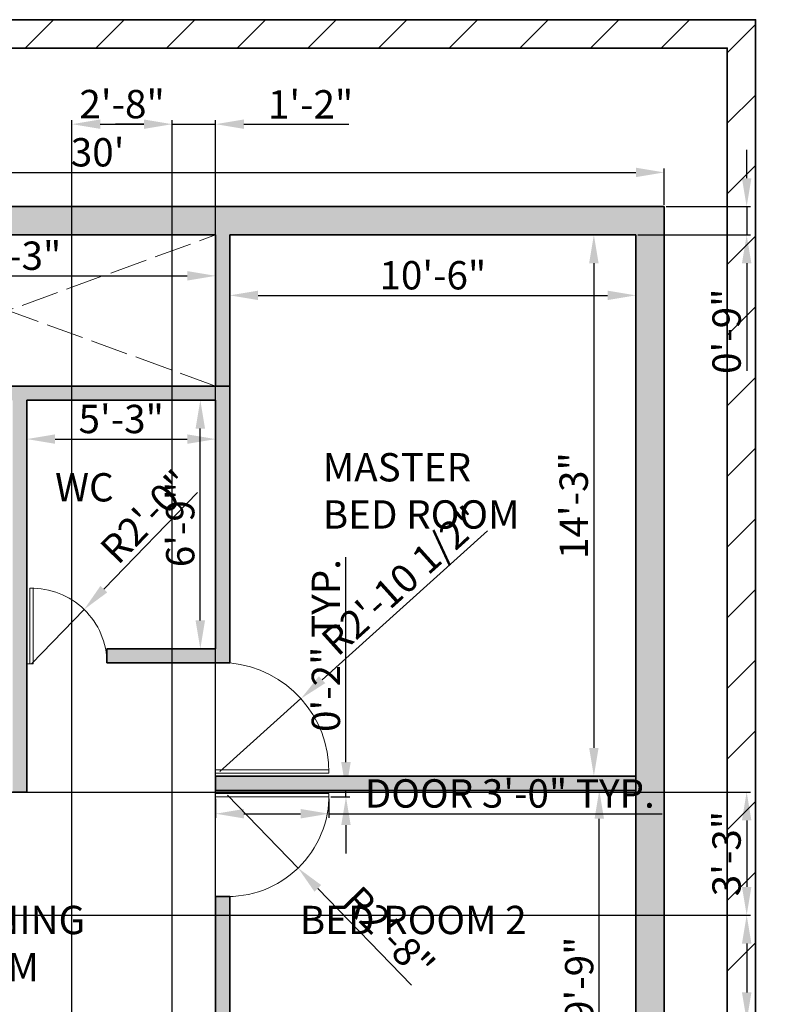
# Model space of a CAD drawing. Units: inches. Extents: x 1130698 to 1131150, y 432269 to 432875.
# Tile 3 of 3: x 1130911 to 1131150, y 432551 to 432864. Entities that reach past the tile are written whole.
import ezdxf

# ---------------------------------------------------------------- set-up
doc = ezdxf.new("R2010")
doc.units = ezdxf.units.IN
doc.linetypes.add('ACAD_ISO02W100', pattern=[15, 12, -3])
for name, color, linetype, lineweight in [('A-ANNO-DIMS', 2, 'Continuous', 18), ('A-ANNO-TTLB', 7, 'Continuous', 35), ('A-AREA-IDEN', 7, 'Continuous', 25), ('A-DOOR', 4, 'Continuous', 18), ('A-ROOF-OVHD', 8, 'ACAD_ISO02W100', 13), ('A-WALL', 7, 'Continuous', 35)]:
    doc.layers.add(name, color=color, linetype=linetype, lineweight=lineweight)
doc.layers.add('A-ANNO-TTLB-PATT', color=251, linetype='Continuous', lineweight=13, true_color=0x636466)
doc.layers.add('A-WALL-PATT', color=251, linetype='Continuous', lineweight=13, true_color=0x636466)
doc.styles.get("Standard").update_dxf_attribs({"font": 'arial.ttf'})
doc.dimstyles.new('ISO-25', dxfattribs={"dimtxt": 9, "dimasz": 9, "dimexe": 1.25, "dimexo": 0.625, "dimtad": 1, "dimdec": 1, "dimrnd": 9, "dimlunit": 3, "dimtxsty": 'Standard', "dimcen": 2.5, "dimadec": 0, "dimazin": 0, "dimtfac": 1, "dimtdec": 1, "dimtmove": 0, "dimatfit": 3, "dimfxl": 1, "dimarcsym": 0})

# ---------------------------------------------------------------- blocks, each defined once
blk = doc.blocks.new('*D3')
at = {"layer": 'A-ANNO-DIMS', "color": 0, "lineweight": -2, "transparency": 16777216}
for p, q in [((1130841.25, 432794.98), (1130841.25, 432781.37)), ((1130973.25, 432794.98), (1130973.25, 432781.37)), ((1130850.25, 432782.62), (1130964.25, 432782.62))]:
    blk.add_line(p, q, dxfattribs=at)
at = {"layer": 'A-ANNO-DIMS', "color": 0, "transparency": 16777216}
for points in [[(1130850.25, 432784.12), (1130850.25, 432781.12), (1130841.25, 432782.62)], [(1130964.25, 432784.12), (1130964.25, 432781.12), (1130973.25, 432782.62)]]:
    blk.add_solid(points, dxfattribs=at)
at = {"layer": 'Defpoints', "color": 0, "transparency": 16777216}
for p in [(1130841.25, 432795.61), (1130973.25, 432795.61), (1130973.25, 432782.62)]:
    blk.add_point(p, dxfattribs=at)
at = {"layer": 'A-ANNO-DIMS', "color": 0, "transparency": 16777216, "insert": (1130907.25, 432787.85), "char_height": 9, "attachment_point": 5}
blk.add_mtext('11\'-3"', dxfattribs=at)
blk = doc.blocks.new('*D5')
at = {"layer": 'A-ANNO-DIMS', "color": 0, "lineweight": -2, "transparency": 16777216}
for p, q in [((1130977.75, 432794.98), (1130977.75, 432775.17)), ((1131106.75, 432794.98), (1131106.75, 432775.17)), ((1130986.75, 432776.42), (1131097.75, 432776.42))]:
    blk.add_line(p, q, dxfattribs=at)
at = {"layer": 'A-ANNO-DIMS', "color": 0, "transparency": 16777216}
for points in [[(1130986.75, 432777.92), (1130986.75, 432774.92), (1130977.75, 432776.42)], [(1131097.75, 432777.92), (1131097.75, 432774.92), (1131106.75, 432776.42)]]:
    blk.add_solid(points, dxfattribs=at)
at = {"layer": 'Defpoints', "color": 0, "transparency": 16777216}
for p in [(1130977.75, 432795.61), (1131106.75, 432795.61), (1131106.75, 432776.42)]:
    blk.add_point(p, dxfattribs=at)
at = {"layer": 'A-ANNO-DIMS', "color": 0, "transparency": 16777216, "insert": (1131042.25, 432781.64), "char_height": 9, "attachment_point": 5}
blk.add_mtext('10\'-6"', dxfattribs=at)
blk = doc.blocks.new('*D6')
at = {"layer": 'A-ANNO-DIMS', "color": 0, "lineweight": -2, "transparency": 16777216}
for p, q in [((1131106.12, 432795.61), (1131092.15, 432795.61)), ((1131093.4, 432786.61), (1131093.4, 432632.61)), ((1131106.12, 432623.61), (1131092.15, 432623.61))]:
    blk.add_line(p, q, dxfattribs=at)
at = {"layer": 'A-ANNO-DIMS', "color": 0, "transparency": 16777216}
for points in [[(1131091.9, 432786.61), (1131094.9, 432786.61), (1131093.4, 432795.61)], [(1131091.9, 432632.61), (1131094.9, 432632.61), (1131093.4, 432623.61)]]:
    blk.add_solid(points, dxfattribs=at)
at = {"layer": 'Defpoints', "color": 0, "transparency": 16777216}
for p in [(1131106.75, 432795.61), (1131093.4, 432623.61), (1131106.75, 432623.61)]:
    blk.add_point(p, dxfattribs=at)
at = {"layer": 'A-ANNO-DIMS', "color": 0, "transparency": 16777216, "insert": (1131088.17, 432709.61), "char_height": 9, "attachment_point": 5, "rotation": 90}
blk.add_mtext('14\'-3"', dxfattribs=at)
blk = doc.blocks.new('*D9')
at = {"layer": 'A-ANNO-DIMS', "color": 0, "lineweight": -2, "transparency": 16777216}
for p, q in [((1130913.25, 432742.48), (1130913.25, 432729.5)), ((1130973.25, 432742.48), (1130973.25, 432729.5)), ((1130922.25, 432730.75), (1130964.25, 432730.75))]:
    blk.add_line(p, q, dxfattribs=at)
at = {"layer": 'A-ANNO-DIMS', "color": 0, "transparency": 16777216}
for points in [[(1130922.25, 432732.25), (1130922.25, 432729.25), (1130913.25, 432730.75)], [(1130964.25, 432732.25), (1130964.25, 432729.25), (1130973.25, 432730.75)]]:
    blk.add_solid(points, dxfattribs=at)
at = {"layer": 'Defpoints', "color": 0, "transparency": 16777216}
for p in [(1130913.25, 432743.11), (1130973.25, 432743.11), (1130973.25, 432730.75)]:
    blk.add_point(p, dxfattribs=at)
at = {"layer": 'A-ANNO-DIMS', "color": 0, "transparency": 16777216, "insert": (1130943.25, 432735.97), "char_height": 9, "attachment_point": 5}
blk.add_mtext('5\'-3"', dxfattribs=at)
blk = doc.blocks.new('*D10')
at = {"layer": 'A-ANNO-DIMS', "color": 0, "lineweight": -2, "transparency": 16777216}
for p, q in [((1130972.62, 432743.11), (1130967.13, 432743.11)), ((1130968.38, 432673.11), (1130968.38, 432734.11)), ((1130972.62, 432664.11), (1130967.13, 432664.11))]:
    blk.add_line(p, q, dxfattribs=at)
at = {"layer": 'A-ANNO-DIMS', "color": 0, "transparency": 16777216}
for points in [[(1130966.88, 432734.11), (1130969.88, 432734.11), (1130968.38, 432743.11)], [(1130966.88, 432673.11), (1130969.88, 432673.11), (1130968.38, 432664.11)]]:
    blk.add_solid(points, dxfattribs=at)
at = {"layer": 'Defpoints', "color": 0, "transparency": 16777216}
for p in [(1130968.38, 432743.11), (1130973.25, 432743.11), (1130973.25, 432664.11)]:
    blk.add_point(p, dxfattribs=at)
at = {"layer": 'A-ANNO-DIMS', "color": 0, "transparency": 16777216, "insert": (1130963.16, 432703.61), "char_height": 9, "attachment_point": 5, "rotation": 90}
blk.add_mtext('6\'-9"', dxfattribs=at)
blk = doc.blocks.new('*D12')
at = {"layer": 'A-ANNO-DIMS', "color": 0, "lineweight": -2, "transparency": 16777216}
for p, q in [((1131106.12, 432619.11), (1131093.87, 432619.11)), ((1131095.12, 432508.11), (1131095.12, 432610.11)), ((1131106.12, 432499.11), (1131093.87, 432499.11))]:
    blk.add_line(p, q, dxfattribs=at)
at = {"layer": 'A-ANNO-DIMS', "color": 0, "transparency": 16777216}
for points in [[(1131093.62, 432610.11), (1131096.62, 432610.11), (1131095.12, 432619.11)], [(1131093.62, 432508.11), (1131096.62, 432508.11), (1131095.12, 432499.11)]]:
    blk.add_solid(points, dxfattribs=at)
at = {"layer": 'Defpoints', "color": 0, "transparency": 16777216}
for p in [(1131095.12, 432619.11), (1131106.75, 432619.11), (1131106.75, 432499.11)]:
    blk.add_point(p, dxfattribs=at)
at = {"layer": 'A-ANNO-DIMS', "color": 0, "transparency": 16777216, "insert": (1131089.9, 432559.11), "char_height": 9, "attachment_point": 5, "rotation": 90}
blk.add_mtext('9\'-9"', dxfattribs=at)
blk = doc.blocks.new('*D20')
at = {"layer": 'A-ANNO-DIMS', "color": 0, "lineweight": -2, "transparency": 16777216}
for p, q in [((1130755.75, 432805.23), (1130755.75, 432816.73)), ((1131115.75, 432805.23), (1131115.75, 432816.73)), ((1130764.75, 432815.48), (1131106.75, 432815.48))]:
    blk.add_line(p, q, dxfattribs=at)
at = {"layer": 'A-ANNO-DIMS', "color": 0, "transparency": 16777216}
for points in [[(1130764.75, 432816.98), (1130764.75, 432813.98), (1130755.75, 432815.48)], [(1131106.75, 432816.98), (1131106.75, 432813.98), (1131115.75, 432815.48)]]:
    blk.add_solid(points, dxfattribs=at)
at = {"layer": 'Defpoints', "color": 0, "transparency": 16777216}
for p in [(1131115.75, 432815.48), (1130755.75, 432804.61), (1131115.75, 432804.61)]:
    blk.add_point(p, dxfattribs=at)
at = {"layer": 'A-ANNO-DIMS', "color": 0, "transparency": 16777216, "insert": (1130935.75, 432820.71), "char_height": 9, "attachment_point": 5}
blk.add_mtext("30'", dxfattribs=at)
blk = doc.blocks.new('DOOR-LEAF-36IN')
for p, q in [((0, 2), (0, 1)), ((0, 1), (36, 1)), ((0, 0), (0, 1)), ((36, 1), (36, 0)), ((36, 0), (0, 0))]:
    blk.add_line(p, q)
blk = doc.blocks.new('DOOR-LEAF-24IN')
for p, q in [((1, 0), (1, 24)), ((1, 24), (2, 24)), ((2, 24), (2, 0)), ((0, 0), (1, 0)), ((2, 0), (1, 0))]:
    blk.add_line(p, q)
blk = doc.blocks.new('*D26')
at = {"layer": 'A-ANNO-DIMS', "color": 0, "lineweight": -2, "transparency": 16777216}
for p, q in [((1130973.25, 432616.48), (1130973.25, 432610.46)), ((1131009.25, 432616.48), (1131009.25, 432610.46)), ((1130982.25, 432611.71), (1131000.25, 432611.71)), ((1131009.25, 432611.71), (1131115.12, 432611.71))]:
    blk.add_line(p, q, dxfattribs=at)
at = {"layer": 'A-ANNO-DIMS', "color": 0, "transparency": 16777216}
for points in [[(1130982.25, 432613.21), (1130982.25, 432610.21), (1130973.25, 432611.71)], [(1131000.25, 432613.21), (1131000.25, 432610.21), (1131009.25, 432611.71)]]:
    blk.add_solid(points, dxfattribs=at)
at = {"layer": 'Defpoints', "color": 0, "transparency": 16777216}
for p in [(1130973.25, 432617.11), (1131009.25, 432617.11), (1131009.25, 432611.71)]:
    blk.add_point(p, dxfattribs=at)
at = {"layer": 'A-ANNO-DIMS', "color": 0, "transparency": 16777216, "insert": (1131066.68, 432616.99), "char_height": 9, "attachment_point": 5}
blk.add_mtext('DOOR 3\'-0" TYP.', dxfattribs=at)
blk = doc.blocks.new('*D27')
at = {"layer": 'A-ANNO-DIMS', "color": 0, "lineweight": -2, "transparency": 16777216}
for p, q in [((1131014.65, 432628.11), (1131014.65, 432693.22)), ((1131009.87, 432619.11), (1131015.9, 432619.11)), ((1131014.65, 432617.11), (1131014.65, 432619.11)), ((1131009.87, 432617.11), (1131015.9, 432617.11)), ((1131014.65, 432608.11), (1131014.65, 432599.11))]:
    blk.add_line(p, q, dxfattribs=at)
at = {"layer": 'A-ANNO-DIMS', "color": 0, "transparency": 16777216}
for points in [[(1131013.15, 432628.11), (1131016.15, 432628.11), (1131014.65, 432619.11)], [(1131013.15, 432608.11), (1131016.15, 432608.11), (1131014.65, 432617.11)]]:
    blk.add_solid(points, dxfattribs=at)
at = {"layer": 'Defpoints', "color": 0, "transparency": 16777216}
for p in [(1131009.25, 432619.11), (1131014.65, 432619.11), (1131009.25, 432617.11)]:
    blk.add_point(p, dxfattribs=at)
at = {"layer": 'A-ANNO-DIMS', "color": 0, "transparency": 16777216, "insert": (1131009.43, 432665.16), "char_height": 9, "attachment_point": 5, "rotation": 90}
blk.add_mtext('0\'-2" TYP.', dxfattribs=at)
blk = doc.blocks.new('*D36')
at = {"layer": 'A-ANNO-DIMS', "color": 0, "lineweight": -2, "transparency": 16777216}
for p, q in [((1130841.96, 432579.47), (1131143.2, 432579.47)), ((1131141.95, 432570.47), (1131141.95, 432554.94)), ((1130842.05, 432545.94), (1131143.2, 432545.94)), ((1131141.95, 432545.94), (1131141.95, 432490.64))]:
    blk.add_line(p, q, dxfattribs=at)
at = {"layer": 'A-ANNO-DIMS', "color": 0, "transparency": 16777216}
for points in [[(1131140.45, 432570.47), (1131143.45, 432570.47), (1131141.95, 432579.47)], [(1131140.45, 432554.94), (1131143.45, 432554.94), (1131141.95, 432545.94)]]:
    blk.add_solid(points, dxfattribs=at)
at = {"layer": 'Defpoints', "color": 0, "transparency": 16777216}
for p in [(1130841.34, 432579.47), (1130841.42, 432545.94), (1131141.95, 432545.94)]:
    blk.add_point(p, dxfattribs=at)
at = {"layer": 'A-ANNO-DIMS', "color": 0, "transparency": 16777216, "insert": (1131136.67, 432513.79), "char_height": 9, "attachment_point": 5, "rotation": 90}
blk.add_mtext('2\'-9 1/2"', dxfattribs=at)
blk = doc.blocks.new('*D37')
at = {"layer": 'A-ANNO-DIMS', "color": 0, "lineweight": -2, "transparency": 16777216}
for p, q in [((1130841.87, 432618.61), (1131143.2, 432618.61)), ((1131141.95, 432609.61), (1131141.95, 432588.47)), ((1130841.96, 432579.47), (1131143.2, 432579.47))]:
    blk.add_line(p, q, dxfattribs=at)
at = {"layer": 'A-ANNO-DIMS', "color": 0, "transparency": 16777216}
for points in [[(1131140.45, 432609.61), (1131143.45, 432609.61), (1131141.95, 432618.61)], [(1131140.45, 432588.47), (1131143.45, 432588.47), (1131141.95, 432579.47)]]:
    blk.add_solid(points, dxfattribs=at)
at = {"layer": 'Defpoints', "color": 0, "transparency": 16777216}
for p in [(1130841.25, 432618.61), (1130841.34, 432579.47), (1131141.95, 432579.47)]:
    blk.add_point(p, dxfattribs=at)
at = {"layer": 'A-ANNO-DIMS', "color": 0, "transparency": 16777216, "insert": (1131136.72, 432599.04), "char_height": 9, "attachment_point": 5, "rotation": 90}
blk.add_mtext('3\'-3"', dxfattribs=at)
blk = doc.blocks.new('*D38')
at = {"layer": 'A-ANNO-DIMS', "color": 0, "lineweight": -2, "transparency": 16777216}
for p, q in [((1130927.61, 432499.23), (1130927.61, 432832.06)), ((1130959.44, 432499.23), (1130959.44, 432832.06)), ((1130936.61, 432830.81), (1130950.44, 432830.81))]:
    blk.add_line(p, q, dxfattribs=at)
at = {"layer": 'A-ANNO-DIMS', "color": 0, "transparency": 16777216}
for points in [[(1130936.61, 432832.31), (1130936.61, 432829.31), (1130927.61, 432830.81)], [(1130950.44, 432832.31), (1130950.44, 432829.31), (1130959.44, 432830.81)]]:
    blk.add_solid(points, dxfattribs=at)
at = {"layer": 'Defpoints', "color": 0, "transparency": 16777216}
for p in [(1130959.44, 432830.81), (1130927.61, 432498.61), (1130959.44, 432498.61)]:
    blk.add_point(p, dxfattribs=at)
at = {"layer": 'A-ANNO-DIMS', "color": 0, "transparency": 16777216, "insert": (1130943.52, 432836.03), "char_height": 9, "attachment_point": 5}
blk.add_mtext('2\'-8"', dxfattribs=at)
blk = doc.blocks.new('*D39')
at = {"layer": 'A-ANNO-DIMS', "color": 0, "lineweight": -2, "transparency": 16777216}
for p, q in [((1130959.44, 432499.23), (1130959.44, 432832.06)), ((1130973.25, 432499.73), (1130973.25, 432832.06)), ((1130950.44, 432830.81), (1130941.44, 432830.81)), ((1130959.44, 432830.81), (1130973.25, 432830.81)), ((1130982.25, 432830.81), (1131015.57, 432830.81))]:
    blk.add_line(p, q, dxfattribs=at)
at = {"layer": 'A-ANNO-DIMS', "color": 0, "transparency": 16777216}
for points in [[(1130950.44, 432832.31), (1130950.44, 432829.31), (1130959.44, 432830.81)], [(1130982.25, 432832.31), (1130982.25, 432829.31), (1130973.25, 432830.81)]]:
    blk.add_solid(points, dxfattribs=at)
at = {"layer": 'Defpoints', "color": 0, "transparency": 16777216}
for p in [(1130973.25, 432830.81), (1130959.44, 432498.61), (1130973.25, 432499.11)]:
    blk.add_point(p, dxfattribs=at)
at = {"layer": 'A-ANNO-DIMS', "color": 0, "transparency": 16777216, "insert": (1131003.41, 432835.95), "char_height": 9, "attachment_point": 5}
blk.add_mtext('1\'-2"', dxfattribs=at)
blk = doc.blocks.new('*D40')
at = {"layer": 'A-ANNO-DIMS', "color": 0, "lineweight": -2, "transparency": 16777216}
for p, q in [((1131141.95, 432813.61), (1131141.95, 432822.61)), ((1131116.37, 432804.61), (1131143.2, 432804.61)), ((1131141.95, 432804.61), (1131141.95, 432795.61)), ((1131107.37, 432795.61), (1131143.2, 432795.61)), ((1131141.95, 432786.61), (1131141.95, 432752.43))]:
    blk.add_line(p, q, dxfattribs=at)
at = {"layer": 'A-ANNO-DIMS', "color": 0, "transparency": 16777216}
for points in [[(1131140.45, 432813.61), (1131143.45, 432813.61), (1131141.95, 432804.61)], [(1131140.45, 432786.61), (1131143.45, 432786.61), (1131141.95, 432795.61)]]:
    blk.add_solid(points, dxfattribs=at)
at = {"layer": 'Defpoints', "color": 0, "transparency": 16777216}
for p in [(1131115.75, 432804.61), (1131106.75, 432795.61), (1131141.95, 432795.61)]:
    blk.add_point(p, dxfattribs=at)
at = {"layer": 'A-ANNO-DIMS', "color": 0, "transparency": 16777216, "insert": (1131136.73, 432765.02), "char_height": 9, "attachment_point": 5, "rotation": 90}
blk.add_mtext('0\'-9"', dxfattribs=at)
blk = doc.blocks.new('*D42')
at = {"layer": 'A-ANNO-DIMS', "color": 0, "lineweight": -2, "transparency": 16777216}
for p, q in [((1131059.64, 432701.63), (1131007.05, 432654.3)), ((1130974.61, 432625.11), (1131000.36, 432648.28))]:
    blk.add_line(p, q, dxfattribs=at)
at = {"layer": 'A-ANNO-DIMS', "color": 0, "transparency": 16777216}
blk.add_solid([(1131006.04, 432655.42), (1131008.05, 432653.19), (1131000.36, 432648.28)], dxfattribs=at)
at = {"layer": 'Defpoints', "color": 0, "transparency": 16777216}
for p in [(1131000.36, 432648.28), (1130974.61, 432625.11)]:
    blk.add_point(p, dxfattribs=at)
at = {"layer": 'A-ANNO-DIMS', "color": 0, "transparency": 16777216, "insert": (1131033.15, 432684.9), "char_height": 9, "attachment_point": 5, "rotation": 41.9872}
blk.add_mtext('R2\'-10 1/2"', dxfattribs=at)
blk = doc.blocks.new('*D45')
at = {"layer": 'A-ANNO-DIMS', "color": 0, "lineweight": -2, "transparency": 16777216}
for p, q in [((1130977.04, 432617.61), (1130999.44, 432594.46)), ((1131035.46, 432557.25), (1131005.7, 432588))]:
    blk.add_line(p, q, dxfattribs=at)
at = {"layer": 'A-ANNO-DIMS', "color": 0, "transparency": 16777216}
blk.add_solid([(1131006.78, 432589.04), (1131004.63, 432586.95), (1130999.44, 432594.46)], dxfattribs=at)
at = {"layer": 'Defpoints', "color": 0, "transparency": 16777216}
for p in [(1130977.04, 432617.61), (1130999.44, 432594.46)]:
    blk.add_point(p, dxfattribs=at)
at = {"layer": 'A-ANNO-DIMS', "color": 0, "transparency": 16777216, "insert": (1131027.46, 432573.02), "char_height": 9, "attachment_point": 5, "rotation": 314.0683}
blk.add_mtext('R2\'-8"', dxfattribs=at)
blk = doc.blocks.new('*D48')
at = {"layer": 'A-ANNO-DIMS', "color": 0, "lineweight": -2, "transparency": 16777216}
for p, q in [((1130967.52, 432713.77), (1130937.72, 432683.06)), ((1130914.75, 432659.39), (1130931.45, 432676.6))]:
    blk.add_line(p, q, dxfattribs=at)
at = {"layer": 'A-ANNO-DIMS', "color": 0, "transparency": 16777216}
blk.add_solid([(1130936.65, 432684.11), (1130938.8, 432682.02), (1130931.45, 432676.6)], dxfattribs=at)
at = {"layer": 'Defpoints', "color": 0, "transparency": 16777216}
for p in [(1130931.45, 432676.6), (1130914.75, 432659.39)]:
    blk.add_point(p, dxfattribs=at)
at = {"layer": 'A-ANNO-DIMS', "color": 0, "transparency": 16777216, "insert": (1130952.01, 432705.28), "char_height": 9, "attachment_point": 5, "rotation": 45.853}
blk.add_mtext('R2\'-0"', dxfattribs=at)

msp = doc.modelspace()

# ---------------------------------------------------------------- hatches: boundary and pattern name
at = {"layer": 'A-ANNO-TTLB-PATT'}
h = msp.add_hatch(dxfattribs=at)
h.set_pattern_fill('ANSI31', color=256, scale=5)
h.paths.add_polyline_path([(1131144.8, 432864.01), (1130698.2, 432864.01), (1130698.2, 432276.41), (1131144.8, 432276.41)])
h.paths.add_polyline_path([(1130707.2, 432855.01), (1131135.8, 432855.01), (1131135.8, 432285.41), (1130707.2, 432285.41)], flags=16)
h.paths.add_polyline_path([(1130755.75, 432804.61), (1131115.75, 432804.61), (1131115.75, 432324.61), (1130908.75, 432324.61), (1130908.75, 432333.61), (1131106.75, 432333.61), (1131106.75, 432494.61), (1131076.75, 432494.61), (1131076.75, 432370.11), (1130908.75, 432370.11), (1130908.75, 432352.4), (1130764.75, 432352.4), (1130764.75, 432333.61), (1130764.75, 432324.61), (1130755.75, 432324.61)], flags=0)
h.paths.add_polyline_path([(1130764.75, 432795.61), (1130836.75, 432795.61), (1130836.75, 432747.61), (1130841.25, 432747.61), (1130841.25, 432795.61), (1130973.25, 432795.61), (1130973.25, 432747.61), (1130977.75, 432747.61), (1130977.75, 432795.61), (1130986.75, 432795.61), (1131106.75, 432795.61), (1131106.75, 432499.11), (1130973.25, 432499.11), (1130973.25, 432498.61), (1130959.44, 432498.61), (1130959.45, 432494.57), (1130973.25, 432494.61), (1131072.25, 432494.61), (1131072.25, 432374.61), (1130913.25, 432374.61), (1130913.25, 432379.9), (1130911, 432379.9), (1130911, 432380.9), (1130911, 432381.9), (1130941, 432381.9, 0.411251), (1130913.25, 432408.94), (1130908.75, 432408.94), (1130908.75, 432498.61), (1130907.75, 432498.61), (1130907.75, 432468.61, -0.386197), (1130873.7, 432498.61), (1130873.7, 432494.37), (1130841.54, 432494.37), (1130841.42, 432545.94), (1130836.75, 432545.94), (1130836.75, 432498.61), (1130764.75, 432498.61), (1130764.75, 432618.61), (1130836.75, 432618.61), (1130836.75, 432579.47), (1130841.34, 432579.47), (1130841.25, 432618.61), (1130874.63, 432618.61), (1130874.63, 432620.86, -0.017137), (1130874.63, 432623.09), (1130874.63, 432623.11), (1130764.75, 432623.11), (1130764.75, 432738.61), (1130764.75, 432743.11), (1130764.75, 432747.61)], flags=0)
h.paths.add_polyline_path([(1130765.75, 432769.36, -0.376584), (1130794.09, 432745.36), (1130794.09, 432743.11), (1130908.75, 432743.11), (1130908.75, 432618.61), (1130913.25, 432618.61), (1130913.25, 432743.11), (1130973.25, 432743.11), (1130973.25, 432664.11), (1130938.73, 432664.11), (1130938.73, 432659.61), (1130977.75, 432659.61, -0.392039), (1131009.25, 432624.61), (1130973.25, 432624.61), (1130973.25, 432623.61), (1130973.25, 432619.11), (1130973.25, 432618.11), (1131009.25, 432618.11, -0.432961), (1130975.5, 432585.44), (1130977.75, 432585.44), (1130977.75, 432585.41, 0.403315), (1131009.25, 432617.11), (1130973.25, 432617.11), (1130973.25, 432618.11), (1130973.25, 432619.11), (1130973.25, 432623.61), (1130973.25, 432624.61), (1130973.25, 432625.61), (1131009.25, 432625.61, 0.383736), (1130977.75, 432659.61), (1130938.73, 432659.61, 0.405522), (1130915.25, 432683.38), (1130915.25, 432659.38), (1130914.25, 432659.38), (1130913.25, 432659.38), (1130913.25, 432618.61), (1130908.75, 432618.61), (1130907.75, 432618.61), (1130906.75, 432618.61), (1130906.75, 432654.61), (1130907.75, 432654.61), (1130907.75, 432618.61), (1130908.75, 432618.61), (1130908.75, 432743.11), (1130794.09, 432743.11), (1130794.09, 432745.36, 0.366478), (1130766.75, 432769.36), (1130766.75, 432745.36), (1130765.75, 432745.36)], flags=0)
h.paths.add_polyline_path([(1130782.75, 432476.15), (1130836.75, 432476.19), (1130836.75, 432458.28), (1130800.75, 432458.19), (1130800.75, 432398.19), (1130812.75, 432398.22), (1130812.75, 432362.22), (1130765.06, 432362.11), (1130782.9, 432380.15)], flags=0)
h.paths.add_polyline_path([(1130794.59, 432383.39), (1130800.75, 432380.15), (1130794.59, 432377.08)], flags=0)
h.paths.add_polyline_path([(1130793.86, 432783.91), (1130807.75, 432783.91), (1130807.75, 432802.46), (1130793.86, 432802.46)], flags=8)
h.paths.add_polyline_path([(1130833.23, 432764.87), (1130833.23, 432778.77), (1130814.69, 432778.77), (1130814.69, 432764.87)], flags=8)
h.paths.add_polyline_path([(1130888.59, 432778.49), (1130925.12, 432778.49), (1130925.12, 432797.04), (1130888.59, 432797.04)], flags=8)
h.paths.add_polyline_path([(1130854.91, 432764.87), (1130854.91, 432778.77), (1130836.36, 432778.77), (1130836.36, 432764.87)], flags=8)
h.paths.add_polyline_path([(1131023.59, 432772.28), (1131060.12, 432772.28), (1131060.12, 432790.83), (1131023.59, 432790.83)], flags=8)
h.paths.add_polyline_path([(1130825.91, 432723.63), (1130846.8, 432723.63), (1130846.8, 432742.18), (1130825.91, 432742.18)], flags=8)
h.paths.add_polyline_path([(1130901.54, 432668.37), (1130901.54, 432697.91), (1130882.99, 432697.91), (1130882.99, 432668.37)], flags=8)
h.paths.add_polyline_path([(1130928.51, 432726.62), (1130958.05, 432726.62), (1130958.05, 432745.17), (1130928.51, 432745.17)], flags=8)
h.paths.add_polyline_path([(1130972.51, 432688.9), (1130972.51, 432718.43), (1130953.97, 432718.43), (1130953.97, 432688.9)], flags=8)
h.paths.add_polyline_path([(1130925.33, 432811.35), (1130946.22, 432811.35), (1130946.22, 432829.9), (1130925.33, 432829.9)], flags=8)
h.paths.add_polyline_path([(1130731.71, 432554.38), (1130731.71, 432575.26), (1130713.17, 432575.26), (1130713.17, 432554.38)], flags=8)
h.paths.add_polyline_path([(1130755.82, 432293.19), (1130947.18, 432293.19), (1130947.18, 432317.92), (1130755.82, 432317.92)], flags=8)
h.paths.add_polyline_path([(1130779.57, 432338.43), (1130829.48, 432338.43), (1130829.48, 432356.98), (1130779.57, 432356.98)], flags=8)
h.paths.add_polyline_path([(1130969.67, 432346.11), (1131010.5, 432346.11), (1131010.5, 432364.66), (1130969.67, 432364.66)], flags=8)
h.paths.add_polyline_path([(1130950.99, 432437.85), (1131016.28, 432437.85), (1131016.28, 432471.55), (1130950.99, 432471.55)], flags=8)
h.paths.add_polyline_path([(1130780.08, 432552.69), (1130839.77, 432552.69), (1130839.77, 432571.24), (1130780.08, 432571.24)], flags=8)
h.paths.add_polyline_path([(1130996.81, 432568.37), (1131080.25, 432568.37), (1131080.25, 432586.92), (1130996.81, 432586.92)], flags=8)
h.paths.add_polyline_path([(1130877.83, 432553.22), (1130935.44, 432553.22), (1130935.44, 432586.93), (1130877.83, 432586.93)], flags=8)
h.paths.add_polyline_path([(1130919.84, 432705.86), (1130945.29, 432705.86), (1130945.29, 432724.41), (1130919.84, 432724.41)], flags=8)
h.paths.add_polyline_path([(1131004.1, 432697.07), (1131077.07, 432697.07), (1131077.07, 432730.77), (1131004.1, 432730.77)], flags=8)
h.paths.add_polyline_path([(1130782.53, 432767.61), (1130807.98, 432767.61), (1130807.98, 432786.15), (1130782.53, 432786.15)], flags=8)
h.paths.add_polyline_path([(1130874.11, 432757.47), (1130904.45, 432757.47), (1130904.45, 432776.02), (1130874.11, 432776.02)], flags=8)
h.paths.add_polyline_path([(1130785.78, 432691.47), (1130858.74, 432691.47), (1130858.74, 432710.01), (1130785.78, 432710.01)], flags=8)
at = {"layer": 'A-WALL-PATT'}
h = msp.add_hatch(color=256, dxfattribs=at)
h.dxf.hatch_style = 1
h.paths.add_polyline_path([(1130764.75, 432738.61), (1130764.75, 432743.11), (1130764.75, 432747.61), (1130764.75, 432795.61), (1130836.75, 432795.61), (1130836.75, 432747.61), (1130841.25, 432747.61), (1130841.25, 432795.61), (1130973.25, 432795.61), (1130973.25, 432747.61), (1130977.75, 432747.61), (1130977.75, 432795.61), (1130986.75, 432795.61), (1131106.75, 432795.61), (1131106.75, 432499.11), (1131106.75, 432494.61), (1131115.75, 432494.61), (1131115.75, 432804.61), (1130755.75, 432804.61), (1130755.75, 432494.37), (1130841.54, 432494.37), (1130841.42, 432545.94), (1130836.75, 432545.94), (1130836.75, 432498.61), (1130764.75, 432498.61), (1130764.75, 432618.61), (1130836.75, 432618.61), (1130836.75, 432579.47), (1130841.34, 432579.47), (1130841.25, 432618.61), (1130874.63, 432618.61), (1130874.63, 432623.11), (1130764.75, 432623.11)])
h.paths.add_polyline_path([(1131106.75, 432623.61), (1130973.25, 432623.61), (1130973.25, 432619.11), (1131106.75, 432619.11)], flags=17)
h.paths.add_polyline_path([(1130913.25, 432743.11), (1130973.25, 432743.11), (1130973.25, 432664.11), (1130938.73, 432664.11), (1130938.73, 432659.61), (1130977.75, 432659.61), (1130977.75, 432743.11), (1130977.75, 432747.61), (1130973.25, 432747.61), (1130794.09, 432747.61), (1130794.09, 432743.11), (1130908.75, 432743.11), (1130908.75, 432618.61), (1130913.25, 432618.61)], flags=17)
h.paths.add_polyline_path([(1131076.75, 432499.11), (1130973.25, 432499.11), (1130973.25, 432498.61), (1130959.44, 432498.61), (1130959.45, 432494.57), (1130973.25, 432494.61), (1131072.25, 432494.61), (1131072.25, 432374.61), (1130913.25, 432374.61), (1130913.25, 432379.9), (1130908.75, 432379.9), (1130908.75, 432370.11), (1131076.75, 432370.11)])
h.paths.add_polyline_path([(1130977.75, 432585.41, -0.017472), (1130975.5, 432585.44), (1130973.25, 432585.44), (1130973.25, 432499.11), (1130977.75, 432499.11)], flags=17)
h.paths.add_polyline_path([(1130873.7, 432498.61), (1130841.53, 432498.61), (1130841.54, 432494.37), (1130873.7, 432494.37)], flags=17)
h.paths.add_polyline_path([(1130913.25, 432494.46), (1130927.62, 432494.5), (1130927.61, 432498.61), (1130908.75, 432498.61), (1130908.75, 432408.94), (1130913.25, 432408.94)])

# ---------------------------------------------------------------- linework, layer by layer
at = {"layer": 'A-ANNO-TTLB'}
for points in [[(1130698.2, 432864.01), (1131144.8, 432864.01), (1131144.8, 432276.41), (1130698.2, 432276.41)], [(1130707.2, 432855.01), (1131135.8, 432855.01), (1131135.8, 432285.41), (1130707.2, 432285.41)]]:
    msp.add_lwpolyline(points, close=True, dxfattribs=at)
at = {"layer": 'A-DOOR'}
for centre, radius, start, end in [((1130914.75, 432659.39), 23.99, 0.5112, 91.1943), ((1130974.61, 432625.11), 34.64, 359.173, 84.8014), ((1130977.04, 432617.61), 32.21, 267.2467, 0.8895)]:
    msp.add_arc(centre, radius, start, end, dxfattribs=at)
at = {"layer": 'A-ROOF-OVHD'}
for p, q in [((1130973.25, 432747.61), (1130841.25, 432795.61)), ((1130841.25, 432747.61), (1130973.25, 432795.61))]:
    msp.add_line(p, q, dxfattribs=at)
at = {"layer": 'A-WALL'}
for p, q in [((1131115.75, 432804.61), (1130755.75, 432804.61)), ((1131115.75, 432324.61), (1131115.75, 432804.61)), ((1130973.25, 432795.61), (1130841.25, 432795.61)), ((1130973.25, 432795.61), (1130973.25, 432747.61)), ((1130986.75, 432795.61), (1130977.75, 432795.61)), ((1130977.75, 432795.61), (1130977.75, 432743.11)), ((1131106.75, 432795.61), (1130986.75, 432795.61)), ((1131106.75, 432499.11), (1131106.75, 432795.61)), ((1130977.75, 432747.61), (1130794.09, 432747.61)), ((1130973.25, 432743.11), (1130913.25, 432743.11)), ((1130913.25, 432743.11), (1130913.25, 432618.61)), ((1130973.25, 432743.11), (1130973.25, 432664.11)), ((1130977.75, 432743.11), (1130977.75, 432659.61)), ((1130973.25, 432664.11), (1130938.73, 432664.11)), ((1130938.73, 432664.11), (1130938.73, 432659.61)), ((1130977.75, 432659.61), (1130938.73, 432659.61)), ((1131106.75, 432623.61), (1130973.25, 432623.61)), ((1130973.25, 432623.61), (1130973.25, 432619.11)), ((1131106.75, 432619.11), (1130973.25, 432619.11)), ((1130913.25, 432618.61), (1130908.75, 432618.61)), ((1130973.25, 432585.44), (1130977.75, 432585.44)), ((1130973.25, 432585.44), (1130973.25, 432498.61)), ((1130977.75, 432585.44), (1130977.75, 432499.11))]:
    msp.add_line(p, q, dxfattribs=at)

# ---------------------------------------------------------------- block references
at = {"layer": 'A-DOOR'}
for name, p in [('DOOR-LEAF-24IN', (1130913.25, 432659.37)), ('DOOR-LEAF-36IN', (1130973.25, 432617.11))]:
    msp.add_blockref(name, p, dxfattribs=at)
at = {"layer": 'A-DOOR', "extrusion": (0, 0, -1), "zscale": -1, "rotation": 180}
msp.add_blockref('DOOR-LEAF-36IN', (-1130973.25, 432625.61), dxfattribs=at)

# ---------------------------------------------------------------- texts
at = {"layer": 'A-AREA-IDEN', "char_height": 9, "attachment_point": 1}
for s, insert in [('MASTER \\PBED ROOM', (1131007.28, 432726.3)), ('WC', (1130922.24, 432719.93)), ('DINNING\\PROOM', (1130881.07, 432582.45)), ('BED ROOM 2', (1130999.98, 432582.45))]:
    msp.add_mtext_dynamic_manual_height_columns(s, width=84.4356, gutter_width=12.5, heights=[0], dxfattribs=dict(at, insert=insert))

# ---------------------------------------------------------------- dimensions: what is measured, and where the dimension line sits
at = {"layer": 'A-ANNO-DIMS'}
for base, p1, p2, override, picture, middle in [((1130959.44, 432830.81), (1130927.61, 432498.61), (1130959.44, 432498.61), {"dimdec": 1, "dimlfac": 1, "dimrnd": 0, "dimzin": 1, "dimdsep": 46, "dimlunit": 4, "dimfrac": 2}, '*D38', (1130943.52, 432836.03)), ((1130973.25, 432830.81), (1130959.44, 432498.61), (1130973.25, 432499.11), {"dimdec": 1, "dimlfac": 1, "dimrnd": 0, "dimzin": 1, "dimdsep": 46, "dimlunit": 4, "dimfrac": 2}, '*D39', (1131003.41, 432835.95)), ((1131115.75, 432815.48), (1130755.75, 432804.61), (1131115.75, 432804.61), {"dimclrd": 0, "dimclre": 0, "dimclrt": 0}, '*D20', (1130935.75, 432820.71)), ((1130973.25, 432782.62), (1130841.25, 432795.61), (1130973.25, 432795.61), {"dimclrd": 0, "dimclre": 0, "dimclrt": 0}, '*D3', (1130907.25, 432787.85)), ((1131106.75, 432776.42), (1130977.75, 432795.61), (1131106.75, 432795.61), {"dimclrd": 0, "dimclre": 0, "dimclrt": 0}, '*D5', (1131042.25, 432781.64)), ((1130973.25, 432730.75), (1130913.25, 432743.11), (1130973.25, 432743.11), {"dimclrd": 0, "dimclre": 0, "dimclrt": 0}, '*D9', (1130943.25, 432735.97))]:
    dim = msp.add_linear_dim(base=base, p1=p1, p2=p2, dimstyle='ISO-25', override=override, dxfattribs=at)
    dim.commit()
    dim.dimension.update_dxf_attribs({"geometry": picture, "text_midpoint": middle})
for base, p1, p2, override, picture, middle in [((1131141.95, 432795.61), (1131115.75, 432804.61), (1131106.75, 432795.61), {"dimdec": 1, "dimlfac": 1, "dimrnd": 0, "dimzin": 1, "dimdsep": 46, "dimlunit": 4, "dimfrac": 2}, '*D40', (1131136.73, 432765.02)), ((1131093.4, 432623.61), (1131106.75, 432795.61), (1131106.75, 432623.61), {"dimclrd": 0, "dimclre": 0, "dimclrt": 0}, '*D6', (1131088.17, 432709.61)), ((1130968.38, 432743.11), (1130973.25, 432664.11), (1130973.25, 432743.11), {"dimclrd": 0, "dimclre": 0, "dimclrt": 0}, '*D10', (1130963.16, 432703.61)), ((1131095.12, 432619.11), (1131106.75, 432499.11), (1131106.75, 432619.11), {"dimclrd": 0, "dimclre": 0, "dimclrt": 0}, '*D12', (1131089.9, 432559.11)), ((1131141.95, 432579.47), (1130841.25, 432618.61), (1130841.34, 432579.47), {"dimdec": 1, "dimlfac": 1, "dimrnd": 0, "dimzin": 1, "dimdsep": 46, "dimlunit": 4, "dimfrac": 2}, '*D37', (1131136.72, 432599.04)), ((1131141.95, 432545.94), (1130841.34, 432579.47), (1130841.42, 432545.94), {"dimdec": 1, "dimlfac": 1, "dimrnd": 0, "dimzin": 1, "dimdsep": 46, "dimlunit": 4, "dimfrac": 2}, '*D36', (1131136.67, 432513.79))]:
    dim = msp.add_linear_dim(base=base, p1=p1, p2=p2, angle=90, dimstyle='ISO-25', override=override, dxfattribs=at)
    dim.commit()
    dim.dimension.update_dxf_attribs({"geometry": picture, "text_midpoint": middle})
for center, mpoint, picture, middle in [((1130914.75, 432659.39), (1130931.45, 432676.6), '*D48', (1130952.01, 432705.28)), ((1130974.61, 432625.11), (1131000.36, 432648.28), '*D42', (1131033.15, 432684.9)), ((1130977.04, 432617.61), (1130999.44, 432594.46), '*D45', (1131027.46, 432573.02))]:
    dim = msp.add_radius_dim(center=center, mpoint=mpoint, dimstyle='ISO-25', override={"dimdec": 1, "dimlfac": 1, "dimrnd": 0, "dimzin": 1, "dimdsep": 46, "dimlunit": 4, "dimfrac": 2}, dxfattribs=at)
    dim.commit()
    dim.dimension.update_dxf_attribs({"geometry": picture, "text_midpoint": middle})
dim = msp.add_linear_dim(base=(1131014.65, 432619.11), p1=(1131009.25, 432617.11), p2=(1131009.25, 432619.11), angle=90, text='<> TYP.', dimstyle='ISO-25', override={"dimdec": 1, "dimlfac": 1, "dimrnd": 0, "dimzin": 1, "dimdsep": 46, "dimlunit": 4, "dimfrac": 2}, dxfattribs=at)
dim.commit()
dim.dimension.update_dxf_attribs({"geometry": '*D27', "text_midpoint": (1131009.43, 432665.16)})
dim = msp.add_linear_dim(base=(1131009.25, 432611.71), p1=(1130973.25, 432617.11), p2=(1131009.25, 432617.11), text='DOOR <> TYP.', dimstyle='ISO-25', override={"dimdec": 1, "dimlfac": 1, "dimrnd": 0, "dimzin": 1, "dimdsep": 46, "dimlunit": 4, "dimfrac": 2}, dxfattribs=at)
dim.commit()
dim.dimension.update_dxf_attribs({"geometry": '*D26', "text_midpoint": (1131066.68, 432616.99)})

doc.saveas('drawing.dxf')
